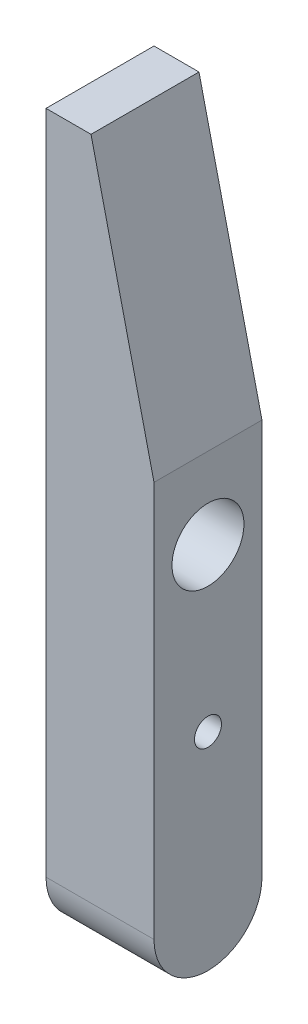
SolidWorks part; units mm, degrees
material "Plain Carbon Steel"
ref_plane "Front Plane" through (0, 0, 0) normal (0, 0, 1) x (1, 0, 0)
ref_plane "Top Plane" through (0, 0, 0) normal (0, 1, 0) x (1, 0, 0)
ref_plane "Right Plane" through (0, 0, 0) normal (1, 0, 0) x (0, 0, -1)
sketch "Jaw Profile Sketch" plane through (0, 0, 0) normal (0, 0, 1) x (1, 0, 0)
  line L0 (0, 0) -> (5, 0)
  line L1 (5, 0) -> (12, -30)
  line L2 (12, -30) -> (12, -74)
  line L3 (12, -74) -> (0, -74)
  line L4 (0, -74) -> (0, 0)
  dimension "D1" = 5
  dimension "D2" = 30
  dimension "D3" = 74
  dimension "D4" = 12
extrude "Jaw Body 12mm" add sketch "Jaw Profile Sketch" along normal mid plane 12
sketch "End Boss Sketch" plane through (0, 0, 0) normal (-1, 0, 0) x (0, 0, 1)
  line L0 (6, -74) -> (-6, -74) construction
  circle A0 centre (0, -74) radius 6
extrude "End Boss" add sketch "End Boss Sketch" against normal up to surface (12 mm away) up to face at (12, -52, 0)
sketch "Cut Ø4.8 Sketch" plane through (0, 0, 0) normal (-1, 0, 0) x (0, 0, 1)
  circle A0 centre (0, -74) radius 2.4
  dimension "D1" = 4.8
extrude "Cut Ø4.8 x 6" cut sketch "Cut Ø4.8 Sketch" against normal blind 6
sketch "Tapped Hole Locations Sketch" plane through (12, 0, 0) normal (1, 0, 0) x (0, 0, -1)
  line L0 (0, -30) -> (0, -80) construction
  line L1 (-6, -30) -> (6, -30) construction
  arc A0 (-6, -74) -> (6, -74) centre (0, -74) ccw construction
  point P7 (0, -74)
hole_wizard "Tapped Hole M8x1.25" positions "3DSketch1" profile "Sketch5" tap size "M8x1.25" standard "ANSI Metric"
sketch3d "3DSketch1"
  line L0 (12, -30, 0) -> (12, -80, 0) construction
  point P0 (12, -39, 0)
  dimension "D1" = 35
sketch "Sketch5" plane through (12, -39, 0) normal (0, 1, 0) x (0, 0, -1)
  line L0 (0, 0) -> (0, 22.1534)
  line L1 (0, 22.1534) -> (4, 19.75)
  line L2 (4, 19.75) -> (4, 0)
  line L5 (4, 0) -> (0, 0)
  line L10 (0, 22.1534) -> (-4, 19.75) construction
  line L11 (0, -6.35) -> (0, 107.95) construction
  dimension "Tap Drill Dia." = 8
  dimension "Tap Drill Depth" = 19.75
  dimension "Drill Angle" = 118
hole_wizard "Tapped Hole M3x0.5" positions "3DSketch2" profile "Sketch6" tap size "M3x0.5" standard "ANSI Metric"
sketch3d "3DSketch2"
  line L0 (12, -30, 0) -> (12, -80, 0) construction
  point P0 (12, -57, 0)
  dimension "D1" = 17
sketch "Sketch6" plane through (12, -57, 0) normal (0, 1, 0) x (0, 0, -1)
  line L0 (0, 0) -> (0, 8.9013)
  line L1 (0, 8.9013) -> (1.5, 8)
  line L2 (1.5, 8) -> (1.5, 0)
  line L5 (1.5, 0) -> (0, 0)
  line L10 (0, 8.9013) -> (-1.5, 8) construction
  line L11 (0, -6.35) -> (0, 107.95) construction
  dimension "Tap Drill Dia." = 3
  dimension "Tap Drill Depth" = 8
  dimension "Drill Angle" = 118
cosmetic thread "Hole Thread1" parameters "D1"=6, "D2"=3
